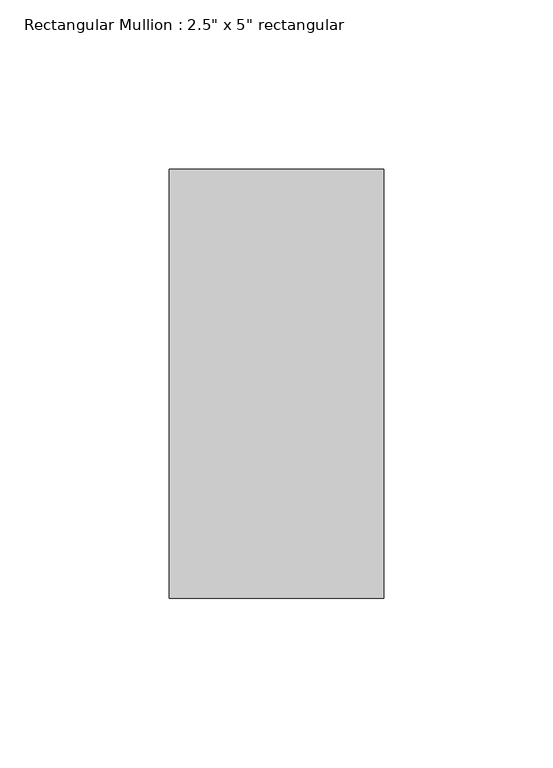
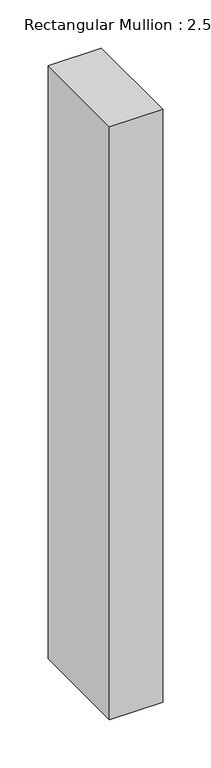
"""IFC4 building model written with IfcOpenShell, lengths in millimetres: member geometry."""

from ifc_helpers import new_model, si_unit, frame, origin, place, context, project, spatial, polyline, outline, extrude, source, transform, mapped, element, save


def member_7982986b(model_context):
    return source(origin(), model_context, "Body", "SweptSolid", [
        extrude(outline(polyline([(31.75, 63.5), (31.75, -63.5), (-31.75, -63.5), (-31.75, 63.5), (31.75, 63.5)])), frame((0.0, 0.0, -750.616916), z_axis=(0.0, 0.0, 1.0), x_axis=(1.0, 0.0, 0.0)), (0.0, 0.0, 1.0), 750.616916),
    ])


if __name__ == "__main__":
    model = new_model("IFC4")
    model_context = context("Model", 3, world=origin())
    ifc_project = project(units=[si_unit("LENGTHUNIT", "METRE", prefix="MILLI")], contexts=[model_context])
    site = spatial("IfcSite", under=ifc_project)
    building = spatial("IfcBuilding", under=site)
    placement = place(None, origin())
    member_shape = member_7982986b(model_context)
    element("IfcMember", 1, ObjectType="Rectangular Mullion : 2.5\" x 5\" rectangular", at=placement, inside=building, context=model_context, shape_type="MappedRepresentation", body=[
        mapped(member_shape, transform((0.0, 0.0, 0.0), x_axis=(1.0, 0.0, 0.0), y_axis=(0.0, 1.0, 0.0), z_axis=(0.0, 0.0, 1.0))),
    ])
    save(model, "model.ifc")

# Revit data of these elements
# Type "Rectangular Mullion : 2.5\" x 5\" rectangular"
#   built-in parameter 1007304 = 0.416667 (stored number, unit not read)
#   built-in parameter 1007301 = 0.104167 (stored number, unit not read)
#   built-in parameter 1007300 = 0.104167 (stored number, unit not read)
# Element 1 (IfcMember, "Rectangular Mullion : 2.5\" x 5\" rectangular")
#   Materials on its faces: "Aluminum"
# Materials
#   "Aluminum": class "Metal", colour RGB 247 247 247, transparency 0, Description = "Aluminum 6061", Cost = 0
